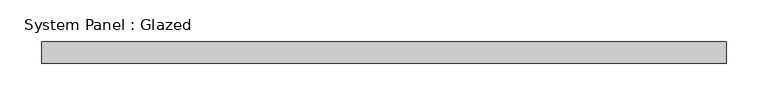
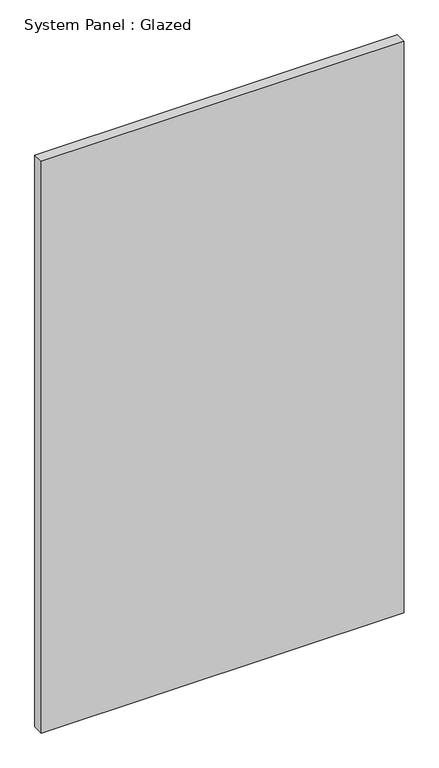
"""IFC4 building model written with IfcOpenShell, lengths in millimetres: plate geometry, System Panel : Glazed."""

from ifc_helpers import new_model, si_unit, origin, origin_with_axes, place, context, project, spatial, polyline, outline, extrude, source, transform, mapped, element, save


def system_panel_glazed_3f785c8f(model_context):
    return source(origin(), model_context, "Body", "SweptSolid", [
        extrude(outline(polyline([(409.575, 19.05), (-409.575, 19.05), (-409.575, 44.45), (409.575, 44.45), (409.575, 19.05)])), origin_with_axes(), (0.0, 0.0, 1.0), 1364.6991558),
    ])


if __name__ == "__main__":
    model = new_model("IFC4")
    model_context = context("Model", 3, world=origin())
    ifc_project = project(units=[si_unit("LENGTHUNIT", "METRE", prefix="MILLI")], contexts=[model_context])
    site = spatial("IfcSite", under=ifc_project)
    building = spatial("IfcBuilding", under=site)
    placement = place(None, origin())
    system_panel_glazed_shape = system_panel_glazed_3f785c8f(model_context)
    element("IfcPlate", 1, ObjectType="System Panel : Glazed", at=placement, inside=building, context=model_context, shape_type="MappedRepresentation", body=[
        mapped(system_panel_glazed_shape, transform((0.0, 0.0, 0.0), x_axis=(1.0, 0.0, 0.0), y_axis=(0.0, 1.0, 0.0), z_axis=(0.0, 0.0, 1.0))),
    ])
    save(model, "model.ifc")

# Revit data of these elements
# Type "System Panel : Glazed"
#   Construction Type Id = "GSP4R"
#   Analytic Construction = "1/8 in Pilkington single glazing"
#   Visual Light Transmittance = 0.9
#   Solar Heat Gain Coefficient = 0.86
#   Heat Transfer Coefficient (U) = 1.18115 BTU/(h·ft²·°F)
#   Define Thermal Properties by = 1
# Element 1 (IfcPlate, "System Panel : Glazed")
#   Materials on its faces: "Glass"
# Materials
#   "Glass": class "Glass", colour RGB 0 128 192, transparency 0.75, Description = "Soda Lime Glass", Cost = 0
